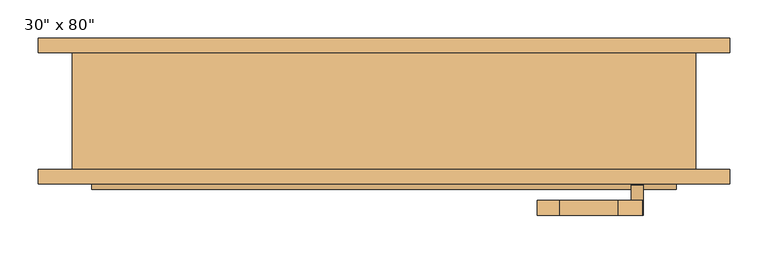
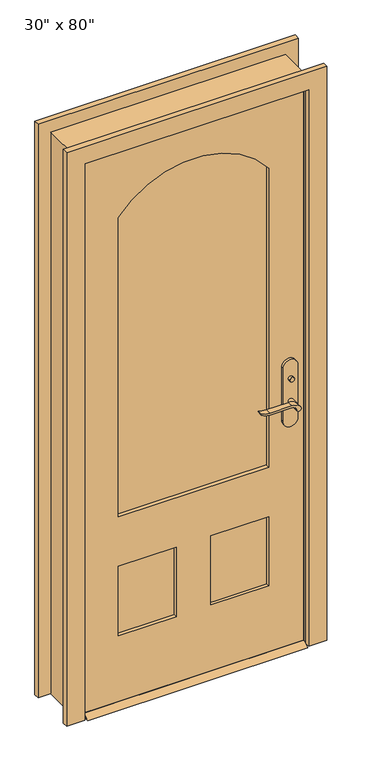
"""IFC4 building model written with IfcOpenShell, lengths in millimetres: door geometry."""

from ifc_helpers import new_model, si_unit, point, frame, frame_2d, origin, place, context, project, spatial, polyline, circle_curve, trimmed, segment, composite_curve, outline, extrude, faceted_brep, source, transform, mapped, element, save


def door_4b146b56(model_context):
    return source(origin(), model_context, "Body", "SolidModel", [
        extrude(outline(polyline([(-38.1, 12.7), (-12.7, 0.0), (-98.425, 0.0), (-73.025, 12.7), (-38.1, 12.7)])), frame((-381.0, 0.0, 0.0), z_axis=(1.0, 0.0, 0.0), x_axis=(0.0, 1.0, 0.0)), (0.0, 0.0, 1.0), 762.0),
        extrude(outline(polyline([(335.2, -18.1), (335.2, -28.1), (325.2, -28.1), (325.2, -18.1), (335.2, -18.1)])), frame((0.0, 0.0, 981.9), z_axis=(0.0, 0.0, 1.0), x_axis=(1.0, 0.0, 0.0)), (0.0, 0.0, 1.0), 30.0),
        extrude(outline(composite_curve([segment(trimmed(circle_curve(frame_2d((996.9, 330.2)), 8.0), [point((996.9, 322.2))], [point((996.9, 338.2))], False, "CARTESIAN"), True, "CONTINUOUS"), segment(trimmed(circle_curve(frame_2d((996.9, 330.2)), 8.0), [point((996.9, 338.2))], [point((996.9, 322.2))], False, "CARTESIAN"), True, "CONTINUOUS")], self_intersect=False)), frame((0.0, -93.025, 0.0), z_axis=(0.0, 1.0, 0.0), x_axis=(0.0, 0.0, 1.0)), (0.0, 0.0, 1.0), 10.0),
        extrude(outline(composite_curve([segment(trimmed(circle_curve(frame_2d((897.1555521, 306.5324871)), 37.2832219), [point((919.0523287, 336.7081363))], [point((934.4, 304.8325667))], False, "CARTESIAN"), True, "CONTINUOUS"), segment(polyline([(934.4, 304.8325667), (934.4, 228.5564091)]), True, "CONTINUOUS"), segment(trimmed(circle_curve(frame_2d((1017.6850638, 228.6227909)), 83.2850902), [point((934.4, 228.5564091))], [point((939.4, 200.2))], True, "CARTESIAN"), True, "CONTINUOUS"), segment(polyline([(939.4, 200.2), (936.6135558, 200.2)]), True, "CONTINUOUS"), segment(trimmed(circle_curve(frame_2d((986.6709207, 232.1396612)), 59.3791355), [point((936.6135558, 200.2))], [point((927.4, 228.5564091))], False, "CARTESIAN"), True, "CONTINUOUS"), segment(polyline([(927.4, 228.5564091), (927.4, 304.8138099)]), True, "CONTINUOUS"), segment(trimmed(circle_curve(frame_2d((909.2738613, 304.8138099)), 18.1261387), [point((927.4, 304.8138099))], [point((914.4, 322.2))], True, "CARTESIAN"), True, "CONTINUOUS"), segment(trimmed(circle_curve(frame_2d((914.4, 330.2)), 8.0), [point((914.4, 322.2))], [point((919.0523287, 336.7081363))], False, "CARTESIAN"), True, "CONTINUOUS")], self_intersect=False)), frame((0.0, 1.9, 0.0), z_axis=(0.0, 1.0, 0.0), x_axis=(0.0, 0.0, 1.0)), (0.0, 0.0, 1.0), 20.0),
        extrude(outline(composite_curve([segment(trimmed(circle_curve(frame_2d((914.4, 330.2)), 8.0), [point((914.3999903, 322.2))], [point((919.0523287, 336.7081363))], False, "CARTESIAN"), True, "CONTINUOUS"), segment(trimmed(circle_curve(frame_2d((897.1555521, 306.5324871)), 37.2832219), [point((919.0523287, 336.7081363))], [point((934.4, 304.8325667))], False, "CARTESIAN"), True, "CONTINUOUS"), segment(polyline([(934.4, 304.8325667), (934.4, 228.5564091)]), True, "CONTINUOUS"), segment(trimmed(circle_curve(frame_2d((1017.6850638, 228.6227909)), 83.2850902), [point((934.4, 228.5564091))], [point((939.4, 200.2))], True, "CARTESIAN"), True, "CONTINUOUS"), segment(polyline([(939.4, 200.2), (936.6135558, 200.2)]), True, "CONTINUOUS"), segment(trimmed(circle_curve(frame_2d((986.6709207, 232.1396612)), 59.3791355), [point((936.6135558, 200.2))], [point((927.4, 228.5564091))], False, "CARTESIAN"), True, "CONTINUOUS"), segment(polyline([(927.4, 228.5564091), (927.4, 304.8138122)]), True, "CONTINUOUS"), segment(trimmed(circle_curve(frame_2d((909.2738682, 304.8138122)), 18.1261318), [point((927.4, 304.8138122))], [point((914.3999903, 322.2))], True, "CARTESIAN"), True, "CONTINUOUS")], self_intersect=False)), frame((0.0, -133.025, 0.0), z_axis=(0.0, 1.0, 0.0), x_axis=(0.0, 0.0, 1.0)), (0.0, 0.0, 1.0), 20.0),
        extrude(outline(composite_curve([segment(trimmed(circle_curve(frame_2d((914.4, 330.2)), 8.0), [point((914.4, 322.2))], [point((914.4, 338.2))], False, "CARTESIAN"), True, "CONTINUOUS"), segment(trimmed(circle_curve(frame_2d((914.4, 330.2)), 8.0), [point((914.4, 338.2))], [point((914.4, 322.2))], False, "CARTESIAN"), True, "CONTINUOUS")], self_intersect=False)), frame((0.0, -28.1, 0.0), z_axis=(0.0, 1.0, 0.0), x_axis=(0.0, 0.0, 1.0)), (0.0, 0.0, 1.0), 30.0),
        extrude(outline(composite_curve([segment(trimmed(circle_curve(frame_2d((914.4, 330.2)), 8.0), [point((914.4, 322.2))], [point((914.4, 338.2))], False, "CARTESIAN"), True, "CONTINUOUS"), segment(trimmed(circle_curve(frame_2d((914.4, 330.2)), 8.0), [point((914.4, 338.2))], [point((914.4, 322.2))], False, "CARTESIAN"), True, "CONTINUOUS")], self_intersect=False)), frame((0.0, -113.025, 0.0), z_axis=(0.0, 1.0, 0.0), x_axis=(0.0, 0.0, 1.0)), (0.0, 0.0, 1.0), 30.0),
        extrude(outline(composite_curve([segment(polyline([(844.4, 355.2), (1039.4, 355.2)]), True, "CONTINUOUS"), segment(trimmed(circle_curve(frame_2d((1039.4, 330.2)), 25.0), [point((1039.4, 355.2))], [point((1039.4, 305.2))], False, "CARTESIAN"), True, "CONTINUOUS"), segment(polyline([(1039.4, 305.2), (844.4, 305.2)]), True, "CONTINUOUS"), segment(trimmed(circle_curve(frame_2d((844.4, 330.2)), 25.0), [point((844.4, 305.2))], [point((844.4, 355.2))], False, "CARTESIAN"), True, "CONTINUOUS")], self_intersect=False)), frame((0.0, -38.1, 0.0), z_axis=(0.0, 1.0, 0.0), x_axis=(0.0, 0.0, 1.0)), (0.0, 0.0, 1.0), 10.0),
        extrude(outline(composite_curve([segment(polyline([(844.4, 355.2), (1039.4, 355.2)]), True, "CONTINUOUS"), segment(trimmed(circle_curve(frame_2d((1039.4, 330.2)), 25.0), [point((1039.4, 355.2))], [point((1039.4, 305.2))], False, "CARTESIAN"), True, "CONTINUOUS"), segment(polyline([(1039.4, 305.2), (844.4, 305.2)]), True, "CONTINUOUS"), segment(trimmed(circle_curve(frame_2d((844.4, 330.2)), 25.0), [point((844.4, 305.2))], [point((844.4, 355.2))], False, "CARTESIAN"), True, "CONTINUOUS")], self_intersect=False)), frame((0.0, -83.025, 0.0), z_axis=(0.0, 1.0, 0.0), x_axis=(0.0, 0.0, 1.0)), (0.0, 0.0, 1.0), 10.0),
        extrude(outline(polyline([(2032.0, -381.0), (12.7, -381.0), (12.7, 381.0), (2032.0, 381.0), (2032.0, -381.0)]), holes=[composite_curve([segment(polyline([(688.975, -260.35), (1784.35, -260.35)]), True, "CONTINUOUS"), segment(trimmed(circle_curve(frame_2d((1580.99125, 0.0)), 330.35875), [point((1784.35, -260.35))], [point((1784.35, 260.35))], True, "CARTESIAN"), True, "CONTINUOUS"), segment(polyline([(1784.35, 260.35), (688.975, 260.35), (688.975, -260.35)]), True, "CONTINUOUS")], self_intersect=False), polyline([(508.0, -60.325), (254.0, -60.325), (254.0, -260.35), (508.0, -260.35), (508.0, -60.325)]), polyline([(508.0, 260.35), (254.0, 260.35), (254.0, 60.325), (508.0, 60.325), (508.0, 260.35)])]), frame((0.0, -73.025, 0.0), z_axis=(0.0, 1.0, 0.0), x_axis=(0.0, 0.0, 1.0)), (0.0, 0.0, 1.0), 34.925),
        faceted_brep([(406.4, -73.025, 0.0), (381.0, -73.025, 0.0), (381.0, -38.1, 0.0), (368.3, -38.1, 0.0), (368.3, -3.175, 0.0), (381.0, -3.175, 0.0), (381.0, 79.375, 0.0), (406.4, 79.375, 0.0), (406.4, 79.375, 2057.4), (406.4, -73.025, 2057.4), (381.0, 79.375, 2032.0), (-381.0, 79.375, 2032.0), (-381.0, 79.375, 0.0), (-406.4, 79.375, 0.0), (-406.4, 79.375, 2057.4), (381.0, -3.175, 2032.0), (368.3, -3.175, 2019.3), (-368.3, -3.175, 2019.3), (-368.3, -3.175, 0.0), (-381.0, -3.175, 0.0), (-381.0, -3.175, 2032.0), (368.3, -38.1, 2019.3), (381.0, -38.1, 2032.0), (-381.0, -38.1, 2032.0), (-381.0, -38.1, 0.0), (-368.3, -38.1, 0.0), (-368.3, -38.1, 2019.3), (381.0, -73.025, 2032.0), (-406.4, -73.025, 2057.4), (-406.4, -73.025, 0.0), (-381.0, -73.025, 0.0), (-381.0, -73.025, 2032.0)], [[[0, 1, 2, 3, 4, 5, 6, 7]], [[7, 8, 9, 0]], [[6, 10, 11, 12, 13, 14, 8, 7]], [[5, 15, 10, 6]], [[4, 16, 17, 18, 19, 20, 15, 5]], [[3, 21, 16, 4]], [[2, 22, 23, 24, 25, 26, 21, 3]], [[1, 27, 22, 2]], [[0, 9, 28, 29, 30, 31, 27, 1]], [[8, 14, 28, 9]], [[15, 20, 11, 10]], [[21, 26, 17, 16]], [[27, 31, 23, 22]], [[29, 13, 12, 19, 18, 25, 24, 30]], [[14, 13, 29, 28]], [[20, 19, 12, 11]], [[26, 25, 18, 17]], [[31, 30, 24, 23]]]),
        extrude(outline(polyline([(-60.325, -49.7416667), (-60.325, -61.3833333), (-260.35, -61.3833333), (-260.35, -49.7416667), (-60.325, -49.7416667)])), frame((0.0, 0.0, 254.0), z_axis=(0.0, 0.0, 1.0), x_axis=(1.0, 0.0, 0.0)), (0.0, 0.0, 1.0), 254.0),
        extrude(outline(polyline([(260.35, -49.7416667), (260.35, -61.3833333), (60.325, -61.3833333), (60.325, -49.7416667), (260.35, -49.7416667)])), frame((0.0, 0.0, 254.0), z_axis=(0.0, 0.0, 1.0), x_axis=(1.0, 0.0, 0.0)), (0.0, 0.0, 1.0), 254.0),
        extrude(outline(composite_curve([segment(polyline([(688.975, -260.35), (688.975, 260.35), (1784.35, 260.35)]), True, "CONTINUOUS"), segment(trimmed(circle_curve(frame_2d((1580.99125, 0.0)), 330.35875), [point((1784.35, 260.35))], [point((1784.35, -260.35))], False, "CARTESIAN"), True, "CONTINUOUS"), segment(polyline([(1784.35, -260.35), (688.975, -260.35)]), True, "CONTINUOUS")], self_intersect=False)), frame((0.0, -59.055, 0.0), z_axis=(0.0, 1.0, 0.0), x_axis=(0.0, 0.0, 1.0)), (0.0, 0.0, 1.0), 6.985),
        extrude(outline(polyline([(0.0, -387.35), (2038.35, -387.35), (2038.35, 387.35), (0.0, 387.35), (0.0, 450.85), (2101.85, 450.85), (2101.85, -450.85), (0.0, -450.85), (0.0, -387.35)])), frame((0.0, 79.375, 0.0), z_axis=(0.0, 1.0, 0.0), x_axis=(0.0, 0.0, 1.0)), (0.0, 0.0, 1.0), 19.05),
        extrude(outline(polyline([(0.0, -387.35), (2038.35, -387.35), (2038.35, 387.35), (0.0, 387.35), (0.0, 450.85), (2101.85, 450.85), (2101.85, -450.85), (0.0, -450.85), (0.0, -387.35)])), frame((0.0, -92.075, 0.0), z_axis=(0.0, 1.0, 0.0), x_axis=(0.0, 0.0, 1.0)), (0.0, 0.0, 1.0), 19.05),
    ])


if __name__ == "__main__":
    model = new_model("IFC4")
    model_context = context("Model", 3, world=origin())
    ifc_project = project(units=[si_unit("LENGTHUNIT", "METRE", prefix="MILLI")], contexts=[model_context])
    site = spatial("IfcSite", under=ifc_project)
    building = spatial("IfcBuilding", under=site)
    placement = place(None, origin())
    door_shape = door_4b146b56(model_context)
    element("IfcDoor", 1, ObjectType="30\" x 80\"", at=placement, inside=building, context=model_context, shape_type="MappedRepresentation", body=[
        mapped(door_shape, transform((0.0, 0.0, 0.0), x_axis=(1.0, 0.0, 0.0), y_axis=(0.0, 1.0, 0.0), z_axis=(0.0, 0.0, 1.0))),
    ])
    save(model, "model.ifc")

# Revit data of these elements
# Type "30\" x 80\""
#   Type Mark = "10"
#   Assembly Code = "B2030100"
#   Analytic Construction = "French door, wood frame with single glass"
#   Threshold Offset [instance default] = 0' - 0 1/2"
#   Thickness = 0' - 1 3/8"
#   Thermal Resistance (R) = 1.0696 (h·ft²·°F)/BTU
#   Swing Angle [instance default] = 90.00°
#   Stiles = 0' - 4 3/4"
#   Rough Width = 2' - 8"
#   Rough Height = 6' - 9"
#   Radius = 1' - 1.00625"
#   Lock Rail = 0' - 7 1/8"
#   Height = 6' - 8"
#   Width = 2' - 6"
#   Heat Transfer Coefficient (U) = 0.9350 BTU/(h·ft²·°F)
#   Door Offset [instance default] = 0' - 0"
#   Bottom Rail = 0' - 9 1/2"
#   Threshold [instance default] = yes
#   Function = 1
#   Exterior Trim [instance default] = yes
#   Trim Material = Cherry
#   Threshold Material = Cherry
#   Panel Material = Cherry
#   Glazing = Glass
#   Frame Material = Cherry
#   Door Handle Material = Aluminum
#   Visual Light Transmittance = 0
#   Solar Heat Gain Coefficient = 0
#   Wall Closure = (empty or 0)
#   Construction Type = (empty or 0)
# Element 1 (IfcDoor, "30\" x 80\"")
#   Materials on its faces: "Cherry", "Aluminum", "Glass"
# Materials
#   "Cherry": class "Wood", colour RGB 226 177 128, transparency 0, Description = "Prunus Serotina", Cost = 0
#   "Glass": class "Glass", colour RGB 0 128 192, transparency 0.75, Description = "Soda Lime Glass", Cost = 0
#   "Aluminum": class "Metal", colour RGB 247 247 247, transparency 0, Description = "Aluminum 6061", Cost = 0
